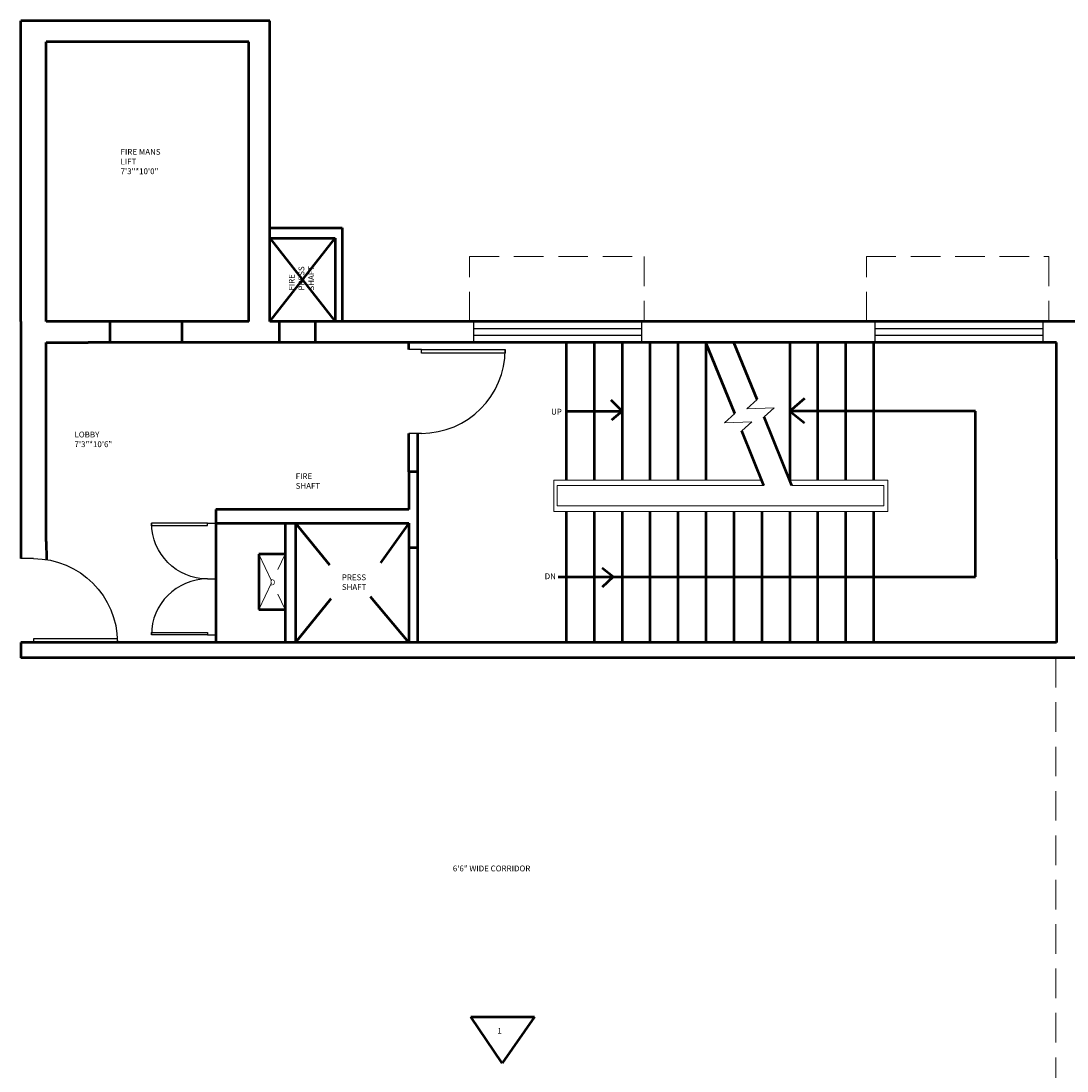
# Model space of a CAD drawing. Units: inches. Extents: x 291 to 2631, y 456 to 2623.
# Tile 6 of 22: x 1014 to 1463, y 934 to 1385. Entities that reach past the tile are written whole.
import ezdxf

# ---------------------------------------------------------------- set-up
doc = ezdxf.new("R2010")
doc.units = ezdxf.units.IN
doc.linetypes.add('DASHED', pattern=[19.05, 12.7, -6.35])
for name, color, linetype, lineweight in [('A-ANNO-TEXT', 3, 'Continuous', 25), ('A-AREA-IDEN', 7, 'Continuous', 25), ('A-DOOR', 3, 'Continuous', 25), ('A-FLOR-OVHD', 1, 'DASHED', 18), ('A-FURN', 8, 'Continuous', 18), ('A-GLAZ', 4, 'Continuous', 25), ('A-WALL', 7, 'Continuous', 50)]:
    doc.layers.add(name, color=color, linetype=linetype, lineweight=lineweight)
doc.styles.get("Standard").update_dxf_attribs({"font": 'arial.ttf'})

# ---------------------------------------------------------------- blocks, each defined once
blk = doc.blocks.new('*U2')
for p, q in [((0, 0), (0, -6)), ((40, 0), (40, -6))]:
    blk.add_line(p, q)
blk.add_lwpolyline([(0, 0), (0, 40), (1.75, 40), (1.75, 0)], close=True)
blk.add_arc((0, 0), 40, 0, 90)
blk = doc.blocks.new('WIN-1800')
for p, q in [((0, 9), (72, 9)), ((0, 0), (0, 9)), ((0, 6), (72, 6)), ((72, 9), (72, 0)), ((72, 3), (0, 3)), ((72, 0), (0, 0))]:
    blk.add_line(p, q)

msp = doc.modelspace()

# ---------------------------------------------------------------- linework, layer by layer
at = {"layer": 'A-FLOR-OVHD'}
for p, q in [((1206.58, 1256.05), (1206.58, 1283.98)), ((1206.58, 1283.98), (1281.55, 1283.98)), ((1281.55, 1283.98), (1281.55, 1256.05)), ((1376.96, 1256.05), (1376.96, 1283.98)), ((1376.96, 1283.98), (1455.3, 1283.98)), ((1455.3, 1283.98), (1455.3, 1256.05)), ((1116.01, 1156.26), (1127.33, 1132.46)), ((1116.01, 1132.46), (1127.33, 1156.26)), ((1458.34, 1111.65), (1458.34, 930.98))]:
    msp.add_line(p, q, dxfattribs=at)
at = {"layer": 'A-FURN'}
for points in [[(1334.74, 1210.84), (1333.01, 1215.1), (1337.35, 1219.02), (1325.66, 1218.58), (1330, 1222.51), (1328.27, 1226.76)], [(1325.85, 1203.18), (1323.45, 1209.11), (1327.78, 1213.03), (1316.1, 1212.6), (1320.43, 1216.52), (1317.41, 1223.96)], [(1344.03, 1188), (1386.13, 1188), (1386.13, 1174.48), (1242.75, 1174.48), (1242.75, 1188), (1332.03, 1188)], [(1344.96, 1185.7), (1384.44, 1185.7), (1384.44, 1176.92), (1244.19, 1176.92), (1244.19, 1185.7), (1332.96, 1185.7)]]:
    msp.add_lwpolyline(points, dxfattribs=at)
at = {"layer": 'A-WALL'}
for p, q in [((1013.95, 1256.05), (1013.95, 1385.05)), ((1120.83, 1385.05), (1013.95, 1385.05)), ((1120.83, 1256.05), (1120.83, 1385.05)), ((1024.83, 1256.05), (1024.83, 1376.05)), ((1111.83, 1376.05), (1024.83, 1376.05)), ((1111.83, 1256.05), (1111.83, 1376.05)), ((1120.83, 1296.25), (1151.9, 1296.25)), ((1151.9, 1296.25), (1151.9, 1256.05)), ((1120.83, 1291.9), (1148.88, 1291.9)), ((1120.83, 1291.9), (1148.88, 1256.05)), ((1120.83, 1256.05), (1148.88, 1291.9)), ((1148.88, 1291.9), (1148.88, 1256.05)), ((1013.95, 1256.05), (1013.95, 1247.05)), ((1042.8, 1256.05), (1024.83, 1256.05)), ((1111.83, 1256.05), (1042.8, 1256.05)), ((1052.16, 1256.05), (1052.16, 1247.05)), ((1082.98, 1256.05), (1082.98, 1247.05)), ((1746.6, 1256.05), (1120.83, 1256.05)), ((1124.82, 1256.05), (1124.82, 1247.05)), ((1140.33, 1256.05), (1140.33, 1247.05)), ((1013.95, 1247.05), (1013.95, 1161.62)), ((1024.83, 1161.62), (1024.83, 1247.05)), ((1024.83, 1247.05), (1042.8, 1247.05)), ((1458.6, 1247.05), (1042.8, 1247.05)), ((1180.47, 1244.05), (1180.47, 1247.05)), ((1248.03, 1247.05), (1248.03, 1188)), ((1260.03, 1247.05), (1260.03, 1188)), ((1272.03, 1247.05), (1272.03, 1188)), ((1284.03, 1247.05), (1284.03, 1188)), ((1296.03, 1247.05), (1296.03, 1188)), ((1308.03, 1247.05), (1308.03, 1188)), ((1320.43, 1216.52), (1308.03, 1247.05)), ((1330, 1222.51), (1320.03, 1247.05)), ((1344.03, 1247.05), (1344.03, 1188)), ((1356.03, 1247.05), (1356.03, 1188)), ((1368.03, 1247.05), (1368.03, 1188)), ((1380.03, 1247.05), (1380.03, 1188)), ((1458.6, 1220), (1458.6, 1247.05)), ((1272.03, 1217.52), (1267.37, 1222.24)), ((1344.03, 1217.52), (1350.58, 1223.15)), ((1248.03, 1217.52), (1272.03, 1217.52)), ((1272.03, 1217.52), (1267.48, 1213.76)), ((1423.85, 1217.52), (1344.03, 1217.52)), ((1344.03, 1217.52), (1350.39, 1212.52)), ((1423.85, 1146.39), (1423.85, 1217.52)), ((1458.6, 1154.05), (1458.6, 1220)), ((1344.96, 1185.7), (1333.01, 1215.1)), ((1180.47, 1191.52), (1180.47, 1208.05)), ((1184.36, 1191.52), (1184.36, 1208.05)), ((1332.96, 1185.7), (1323.45, 1209.11)), ((1184.36, 1191.52), (1180.47, 1191.52)), ((1180.47, 1191.52), (1180.47, 1175.39)), ((1184.36, 1175.39), (1184.36, 1191.52)), ((1180.47, 1175.39), (1097.67, 1175.39)), ((1097.67, 1175.39), (1097.67, 1118.3)), ((1184.36, 1118.3), (1184.36, 1175.39)), ((1248.03, 1174.48), (1248.03, 1118.3)), ((1260.03, 1174.48), (1260.03, 1118.3)), ((1272.03, 1174.48), (1272.03, 1118.3)), ((1284.03, 1174.48), (1284.03, 1118.3)), ((1296.03, 1174.48), (1296.03, 1118.3)), ((1308.03, 1174.48), (1308.03, 1118.3)), ((1320.03, 1174.48), (1320.03, 1118.3)), ((1332.03, 1174.48), (1332.03, 1118.3)), ((1344.03, 1174.48), (1344.03, 1118.3)), ((1356.03, 1174.48), (1356.03, 1118.3)), ((1368.03, 1174.48), (1368.03, 1118.3)), ((1380.03, 1174.48), (1380.03, 1118.3)), ((1097.67, 1169.54), (1175.36, 1169.54)), ((1127.33, 1169.54), (1127.33, 1118.3)), ((1131.77, 1169.54), (1131.77, 1118.3)), ((1131.77, 1169.54), (1146.38, 1151.62)), ((1180.47, 1169.54), (1168.37, 1152.45)), ((1175.36, 1169.54), (1180.47, 1169.54)), ((1180.47, 1169.54), (1180.47, 1118.3)), ((1013.95, 1161.62), (1013.95, 1154.3)), ((1024.83, 1161.62), (1024.84, 1153.88)), ((1180.47, 1159), (1184.36, 1159)), ((1127.33, 1156.26), (1116.01, 1156.26)), ((1116.01, 1156.26), (1116.01, 1132.46)), ((1458.6, 1154.05), (1458.6, 1118.3)), ((1268.17, 1146.39), (1263.54, 1150.2)), ((1244.56, 1146.39), (1423.85, 1146.39)), ((1268.17, 1146.39), (1263.44, 1141.99)), ((1131.77, 1118.3), (1147.08, 1137.19)), ((1180.47, 1118.3), (1164.02, 1137.94)), ((1116.01, 1132.46), (1127.33, 1132.46)), ((1034.19, 1118.3), (1013.95, 1118.3)), ((1013.95, 1118.3), (1013.95, 1111.65)), ((1458.6, 1118.3), (1034.19, 1118.3)), ((1032.82, 1111.65), (1013.95, 1111.65)), ((1467.6, 1111.65), (1032.82, 1111.65)), ((1207.07, 957.64), (1234.46, 957.64)), ((1220.62, 937.71), (1207.07, 957.64)), ((1234.46, 957.64), (1220.62, 937.71))]:
    msp.add_line(p, q, dxfattribs=at)

# ---------------------------------------------------------------- block references
at = {"layer": 'A-DOOR'}
for p, xscale, yscale, zscale, rotation in [((1185.87, 1244.05), 0.9, 0.9, 0.9, 270), ((1094.03, 1169.54), -0.6, 0.6, 0.6, 90), ((1019.35, 1118.3), -0.9, 0.9, 0.9, 270), ((1093.98, 1121.54), 0.6, 0.6, 0.6, 89.99999999999999)]:
    msp.add_blockref('*U2', p, dxfattribs=dict(at, xscale=xscale, yscale=yscale, zscale=zscale, rotation=rotation))
at = {"layer": 'A-GLAZ'}
for p in [(1208.46, 1247.05), (1380.73, 1247.05)]:
    msp.add_blockref('WIN-1800', p, dxfattribs=at)

# ---------------------------------------------------------------- texts
at = {"layer": 'A-ANNO-TEXT', "char_height": 2.5, "attachment_point": 1}
for s, width, insert in [('UP', 11.4241, (1241.56, 1218.59)), ('D', 2.0681, (1120.79, 1145.36)), ('DN', 7.5075, (1238.82, 1147.95)), ('1', 8.9528, (1218.53, 952.86))]:
    msp.add_mtext_dynamic_manual_height_columns(s, width=width, gutter_width=12.5, heights=[0], dxfattribs=dict(at, insert=insert))
at = {"layer": 'A-AREA-IDEN', "char_height": 2.5, "attachment_point": 1}
for s, width, insert in [('FIRE MANS\\PLIFT\\P7\'3"*10\'0"', 59.686, (1056.73, 1330.13)), ('LOBBY\\P7\'3"*10\'6"', 51.4873, (1036.92, 1208.8)), ('FIRE\\PSHAFT', 32.5348, (1131.9, 1190.92)), ('PRESS\\PSHAFT', 22.8902, (1151.73, 1147.49)), ('6\'6" WIDE CORRIDOR', 322.1506, (1199.37, 1022.53))]:
    msp.add_mtext_dynamic_manual_height_columns(s, width=width, gutter_width=12.5, heights=[0], dxfattribs=dict(at, insert=insert))
at = {"layer": 'A-AREA-IDEN', "insert": (1128.96, 1269.35), "char_height": 2.5, "attachment_point": 1, "rotation": 90}
msp.add_mtext_dynamic_manual_height_columns('FIRE\\PPRESS\\PSHAFT', width=23.4589, gutter_width=12.5, heights=[0], dxfattribs=at)

doc.saveas('drawing.dxf')
